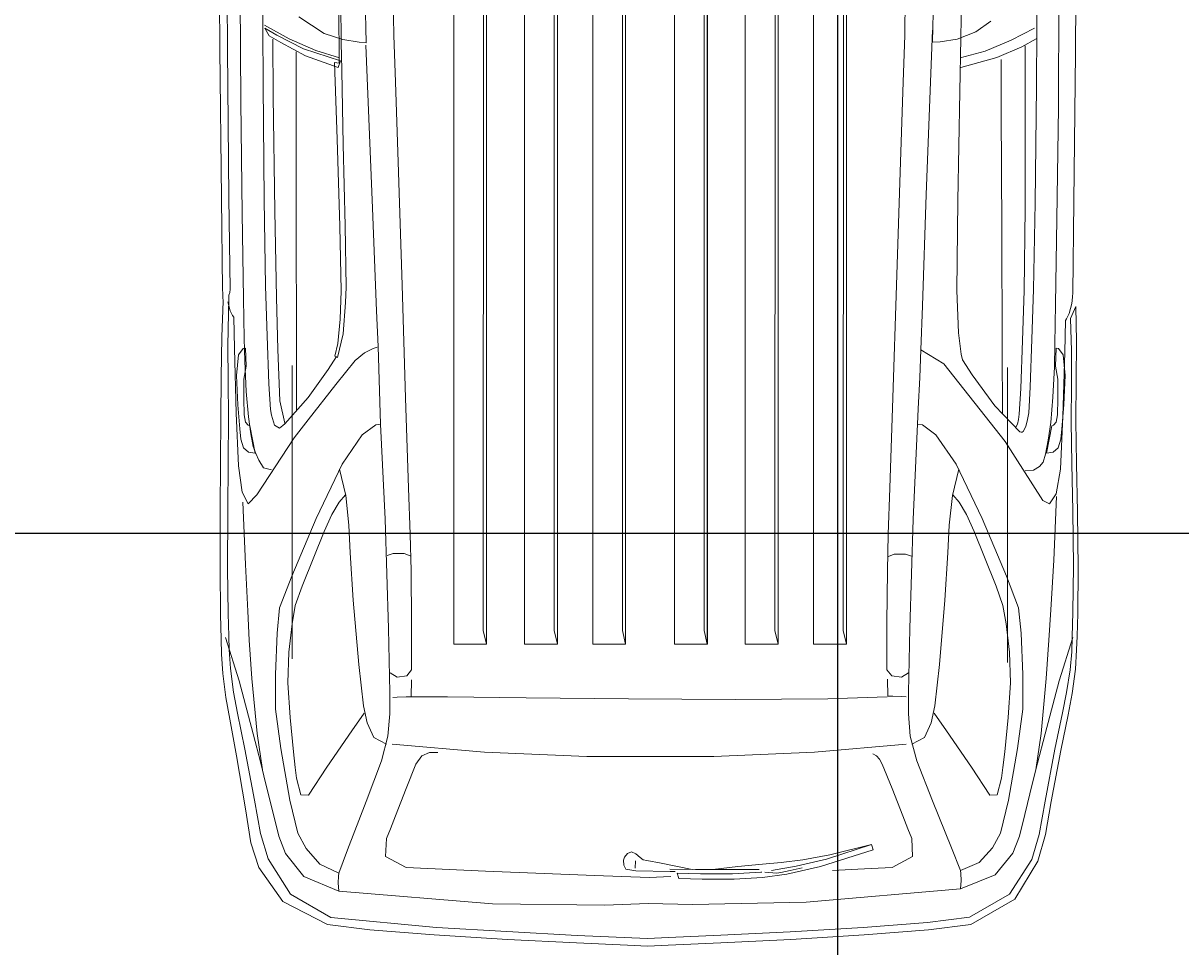
# Model space of a CAD drawing. Units: inches. Extents: x 37 to 706, y -568 to 110.
# Tile 11 of 24: x 444 to 494, y -468 to -428. Entities that reach past the tile are written whole.
import ezdxf

# ---------------------------------------------------------------- set-up
doc = ezdxf.new("R2010")
doc.units = ezdxf.units.IN
doc.header["$MEASUREMENT"] = 0
doc.layers.add('A-ANNO-DIMS', color=2, linetype='Continuous', lineweight=18)
doc.layers.add('A-SITE-VEHI', color=8, linetype='Continuous', lineweight=13)
doc.styles.get("Standard").update_dxf_attribs({"font": 'arial.ttf'})
doc.dimstyles.get("Standard").update_dxf_attribs({"dimtxt": 0.18, "dimasz": 0.18, "dimexe": 0.18, "dimexo": 0.0625, "dimgap": 0.09, "dimtad": 0, "dimtih": 1, "dimtoh": 1, "dimdec": 0, "dimzin": 0, "dimdsep": 46, "dimlunit": 3, "dimtxsty": 'Standard', "dimcen": 0.09, "dimadec": 0, "dimazin": 0, "dimtfac": 1, "dimtdec": 0, "dimtofl": 0, "dimtmove": 0, "dimatfit": 3, "dimfxl": 1, "dimtolj": 1, "dimtzin": 0, "dimarcsym": 0})

# ---------------------------------------------------------------- blocks, each defined once
blk = doc.blocks.new('CAR-SEDAN-PLAN')
for p, q in [((13.604, 13.133), (13.604, 50.661)), ((14.891, 13.73), (14.905, 50.543)), ((15.034, 50.661), (15.034, 13.133)), ((15.035, 50.661), (15.035, 13.133)), ((16.686, 13.133), (16.686, 50.661)), ((17.973, 13.73), (17.987, 50.543)), ((18.115, 50.661), (18.115, 13.133)), ((18.117, 50.661), (18.117, 13.133)), ((19.657, 13.133), (19.657, 50.661)), ((20.944, 13.73), (20.958, 50.543)), ((21.087, 50.661), (21.087, 13.133)), ((21.088, 50.661), (21.088, 13.133)), ((23.212, 13.133), (23.212, 50.661)), ((24.499, 13.73), (24.513, 50.543)), ((24.642, 50.661), (24.642, 13.133)), ((24.643, 50.661), (24.643, 13.133)), ((26.294, 13.133), (26.294, 50.661)), ((27.581, 13.73), (27.595, 50.543)), ((27.723, 50.661), (27.723, 13.133)), ((27.725, 50.661), (27.725, 13.133)), ((29.265, 13.133), (29.265, 50.661)), ((30.553, 13.73), (30.567, 50.543)), ((30.696, 50.661), (30.696, 13.133)), ((9.713, 43.414), (9.796, 39.289)), ((5.287, 43.269), (5.301, 39.967)), ((34.542, 43.262), (34.438, 39.318)), ((35.714, 43.262), (35.681, 39.496)), ((38.971, 43.074), (38.982, 39.925)), ((3.432, 39.004), (3.403, 42.392)), ((3.734, 42.392), (3.762, 39.007)), ((4.314, 41.922), (4.342, 36.731)), ((40.658, 38.847), (40.687, 42.232)), ((10.998, 39.61), (10.962, 41.449)), ((33.232, 39.61), (33.258, 41.449)), ((39.946, 41.674), (39.918, 36.482)), ((8.623, 38.413), (8.61, 40.812)), ((8.689, 40.947), (8.707, 39.376)), ((7.97, 39.706), (6.86, 40.42)), ((5.301, 39.967), (5.315, 37.467)), ((5.378, 40.068), (6.446, 39.47)), ((5.576, 39.596), (5.383, 39.926)), ((5.383, 39.926), (5.907, 39.624)), ((34.436, 39.852), (34.17, 32.694)), ((36.321, 39.78), (36.975, 40.234)), ((38.884, 39.936), (37.863, 39.414)), ((38.982, 39.925), (38.961, 37.396)), ((6.083, 39.306), (5.576, 39.596)), ((5.727, 39.459), (5.754, 36.963)), ((5.907, 39.624), (7.068, 39.031)), ((7.162, 38.735), (6.083, 39.306)), ((6.446, 39.47), (7.6, 38.961)), ((8.786, 39.439), (7.97, 39.706)), ((8.707, 39.376), (8.71, 39.215)), ((9.493, 39.318), (8.786, 39.439)), ((9.796, 39.289), (9.493, 39.318)), ((11.071, 37.604), (10.998, 39.61)), ((33.159, 37.604), (33.232, 39.61)), ((34.438, 39.318), (34.768, 39.333)), ((34.768, 39.333), (35.515, 39.45)), ((35.515, 39.45), (36.321, 39.78)), ((35.681, 39.496), (35.635, 37.18)), ((37.863, 39.414), (36.73, 38.932)), ((38.331, 39.125), (38.947, 39.462)), ((3.493, 32.542), (3.432, 39.004)), ((3.762, 39.007), (3.823, 32.551)), ((6.745, 38.908), (6.755, 31.469)), ((7.068, 39.031), (8.678, 38.516)), ((7.6, 38.961), (8.63, 38.647)), ((8.71, 39.215), (8.718, 38.766)), ((9.785, 39.195), (10.065, 32.102)), ((36.73, 38.932), (35.646, 38.643)), ((37.235, 38.651), (38.331, 39.125)), ((38.468, 39.17), (38.473, 36.823)), ((40.598, 32.392), (40.658, 38.847)), ((8.583, 38.221), (7.162, 38.735)), ((8.528, 35.109), (8.424, 38.44)), ((8.424, 38.44), (8.623, 38.413)), ((8.678, 38.516), (8.583, 38.221)), ((8.718, 38.766), (8.731, 38.071)), ((35.681, 38.217), (37.235, 38.651)), ((37.423, 38.564), (37.433, 36.292)), ((8.731, 38.071), (8.801, 34.877)), ((5.315, 37.467), (5.354, 32.465)), ((11.199, 33.662), (11.071, 37.604)), ((33.03, 33.662), (33.159, 37.604)), ((38.961, 37.396), (38.908, 32.341)), ((5.754, 36.963), (5.818, 31.97)), ((35.635, 37.18), (35.548, 32.425)), ((38.473, 36.823), (38.469, 32.105)), ((4.342, 36.731), (4.403, 31.875)), ((37.433, 36.292), (37.457, 31.221)), ((39.918, 36.482), (39.857, 31.627)), ((8.645, 31.317), (8.528, 35.109)), ((8.801, 34.877), (8.881, 31.335)), ((11.355, 28.753), (11.199, 33.662)), ((32.874, 28.753), (33.03, 33.662)), ((3.546, 28.561), (3.493, 32.542)), ((3.823, 32.551), (3.876, 28.574)), ((5.354, 32.465), (5.415, 28.71)), ((34.17, 32.694), (34.002, 27.855)), ((35.548, 32.425), (35.501, 28.522)), ((38.908, 32.341), (38.84, 28.558)), ((40.545, 28.416), (40.598, 32.392)), ((4.403, 31.875), (4.464, 28.172)), ((5.818, 31.97), (5.892, 28.219)), ((10.065, 32.102), (10.25, 27.635)), ((38.469, 32.105), (38.427, 28.503)), ((6.755, 31.469), (6.762, 26.153)), ((8.713, 28.508), (8.645, 31.317)), ((8.881, 31.335), (8.919, 28.667)), ((39.857, 31.627), (39.796, 27.924)), ((37.457, 31.221), (37.48, 25.971)), ((11.511, 23.847), (11.355, 28.753)), ((32.718, 23.847), (32.874, 28.753)), ((3.551, 28.393), (3.546, 28.561)), ((3.558, 28.225), (3.551, 28.393)), ((3.579, 28.059), (3.558, 28.225)), ((3.819, 28.315), (3.815, 28.178)), ((3.856, 28.436), (3.819, 28.315)), ((3.876, 28.574), (3.856, 28.436)), ((5.415, 28.71), (5.486, 26.554)), ((5.892, 28.219), (5.946, 25.954)), ((8.671, 27.267), (8.713, 28.508)), ((8.919, 28.667), (8.894, 27.992)), ((35.501, 28.522), (35.566, 26.682)), ((38.427, 28.503), (38.356, 26.347)), ((38.84, 28.558), (38.769, 26.402)), ((40.519, 28.091), (40.535, 28.246)), ((40.535, 28.246), (40.545, 28.416)), ((3.52, 26.505), (3.579, 28.059)), ((3.88, 27.64), (3.771, 28.026)), ((3.815, 28.178), (3.801, 27.531)), ((4.464, 28.172), (4.492, 26.437)), ((8.894, 27.992), (8.788, 26.636)), ((34.002, 27.855), (33.939, 25.939)), ((39.796, 27.924), (39.768, 26.188)), ((40.387, 27.519), (40.498, 27.951)), ((40.449, 27.298), (40.675, 27.828)), ((40.498, 27.951), (40.519, 28.091)), ((40.675, 27.828), (40.709, 26.308)), ((3.801, 27.531), (3.77, 26.116)), ((3.984, 27.426), (3.88, 27.64)), ((4.03, 27.36), (3.984, 27.426)), ((4.062, 25.992), (4.03, 27.36)), ((8.558, 26.208), (8.671, 27.267)), ((10.25, 27.635), (10.317, 26.081)), ((40.194, 25.84), (40.225, 27.208)), ((40.225, 27.208), (40.276, 27.281)), ((40.276, 27.281), (40.387, 27.519)), ((40.488, 25.901), (40.449, 27.298)), ((3.484, 24.748), (3.52, 26.505)), ((4.492, 26.437), (4.514, 25.45)), ((5.486, 26.554), (5.557, 24.461)), ((8.437, 25.661), (8.558, 26.208)), ((8.788, 26.636), (8.548, 25.606)), ((35.566, 26.682), (35.686, 25.757)), ((38.356, 26.347), (38.285, 24.254)), ((38.769, 26.402), (38.698, 24.309)), ((40.709, 26.308), (40.697, 24.613)), ((3.77, 26.116), (3.787, 24.613)), ((4.141, 23.187), (4.062, 25.992)), ((4.24, 25.718), (4.151, 24.827)), ((4.44, 26.001), (4.24, 25.718)), ((4.551, 26.018), (4.44, 26.001)), ((4.571, 25.221), (4.551, 26.018)), ((5.946, 25.954), (6.033, 23.727)), ((6.762, 26.153), (6.765, 23.311)), ((9.729, 25.804), (9.322, 25.478)), ((10.107, 25.994), (9.729, 25.804)), ((10.273, 26.055), (10.107, 25.994)), ((10.317, 26.081), (10.426, 22.71)), ((33.939, 25.939), (33.885, 24.736)), ((33.939, 25.939), (34.933, 25.326)), ((35.686, 25.757), (35.75, 25.503)), ((37.48, 25.971), (37.49, 23.159)), ((39.768, 26.188), (39.746, 25.202)), ((39.796, 25.221), (39.816, 26.018)), ((39.816, 26.018), (39.928, 26.001)), ((39.928, 26.001), (40.128, 25.718)), ((40.115, 23.036), (40.194, 25.84)), ((40.128, 25.718), (40.217, 24.827)), ((40.485, 24.433), (40.488, 25.901)), ((4.47, 24.664), (4.571, 25.221)), ((4.514, 25.45), (4.576, 24.132)), ((6.579, 25.262), (6.579, 12.495)), ((8.505, 25.655), (8.139, 25.088)), ((8.548, 25.606), (8.437, 25.661)), ((9.322, 25.478), (8.474, 24.429)), ((34.933, 25.326), (37.597, 21.952)), ((35.75, 25.503), (36.174, 24.851)), ((39.746, 25.202), (39.684, 23.884)), ((39.897, 24.664), (39.796, 25.221)), ((3.472, 22.96), (3.484, 24.748)), ((4.151, 24.827), (4.216, 23.545)), ((8.139, 25.088), (7.271, 23.868)), ((33.885, 24.736), (33.823, 23.365)), ((36.174, 24.851), (37.15, 23.504)), ((37.699, 25.17), (37.699, 12.334)), ((40.217, 24.827), (40.151, 23.545)), ((3.787, 24.613), (3.803, 22.96)), ((4.466, 23.8), (4.47, 24.664)), ((5.557, 24.461), (5.628, 23.347)), ((8.474, 24.429), (7.27, 22.892)), ((38.285, 24.254), (38.214, 23.14)), ((38.698, 24.309), (38.627, 23.195)), ((39.901, 23.8), (39.897, 24.664)), ((40.477, 22.799), (40.485, 24.433)), ((40.697, 24.613), (40.683, 22.854)), ((4.482, 23.116), (4.466, 23.8)), ((4.576, 24.132), (4.669, 23.027)), ((6.033, 23.727), (6.25, 22.744)), ((7.271, 23.868), (6.252, 22.718)), ((11.64, 19.914), (11.511, 23.847)), ((32.59, 19.914), (32.718, 23.847)), ((39.684, 23.884), (39.591, 22.779)), ((39.885, 23.116), (39.901, 23.8)), ((4.243, 20.896), (4.141, 23.187)), ((4.216, 23.545), (4.303, 22.495)), ((5.628, 23.347), (5.675, 23.096)), ((33.823, 23.365), (33.793, 22.71)), ((37.15, 23.504), (38.236, 22.378)), ((38.627, 23.195), (38.57, 22.906)), ((40.151, 23.545), (40.064, 22.495)), ((3.463, 21.075), (3.472, 22.96)), ((3.803, 22.96), (3.793, 21.075)), ((4.546, 22.789), (4.482, 23.116)), ((4.666, 22.658), (4.546, 22.789)), ((4.669, 23.027), (4.776, 22.289)), ((5.675, 23.096), (5.809, 22.664)), ((6.173, 22.65), (6.252, 22.718)), ((7.27, 22.892), (6.658, 22.104)), ((10.426, 22.71), (10.213, 22.669)), ((10.426, 22.71), (10.623, 18.569)), ((33.793, 22.71), (33.596, 18.569)), ((33.793, 22.71), (34.007, 22.669)), ((38.142, 22.707), (38.056, 22.552)), ((38.178, 22.908), (38.142, 22.707)), ((38.214, 23.14), (38.178, 22.908)), ((38.57, 22.906), (38.496, 22.598)), ((39.591, 22.779), (39.479, 22.007)), ((39.702, 22.658), (39.821, 22.789)), ((39.821, 22.789), (39.885, 23.116)), ((40.012, 20.744), (40.115, 23.036)), ((40.502, 20.982), (40.477, 22.799)), ((40.683, 22.854), (40.709, 20.996)), ((4.303, 22.495), (4.347, 22.059)), ((4.73, 22.634), (4.666, 22.658)), ((4.964, 21.437), (4.73, 22.634)), ((4.776, 22.289), (4.883, 21.74)), ((5.809, 22.664), (6.019, 22.53)), ((6.019, 22.53), (6.095, 22.587)), ((6.095, 22.587), (6.173, 22.65)), ((9.627, 22.239), (8.747, 20.959)), ((10.213, 22.669), (9.627, 22.239)), ((34.007, 22.669), (34.593, 22.239)), ((34.593, 22.239), (35.473, 20.959)), ((38.236, 22.378), (38.293, 22.351)), ((38.293, 22.351), (38.344, 22.355)), ((38.344, 22.355), (38.389, 22.385)), ((38.496, 22.598), (38.389, 22.385)), ((39.404, 21.437), (39.637, 22.634)), ((39.637, 22.634), (39.702, 22.658)), ((40.064, 22.495), (40.02, 22.059)), ((4.347, 22.059), (4.458, 21.676)), ((4.458, 21.676), (4.673, 21.491)), ((4.883, 21.74), (4.989, 21.429)), ((6.658, 22.104), (5.04, 19.635)), ((37.597, 21.952), (39.239, 19.387)), ((39.479, 22.007), (39.364, 21.397)), ((39.909, 21.676), (39.695, 21.491)), ((40.02, 22.059), (39.909, 21.676)), ((4.673, 21.491), (4.964, 21.437)), ((4.989, 21.429), (5.122, 21.136)), ((39.364, 21.397), (39.252, 21.052)), ((39.695, 21.491), (39.404, 21.437)), ((3.446, 18.903), (3.463, 21.075)), ((3.793, 21.075), (3.776, 18.903)), ((4.396, 19.749), (4.243, 20.896)), ((5.122, 21.136), (5.335, 20.805)), ((5.335, 20.805), (5.672, 20.722)), ((8.747, 20.959), (7.622, 18.6)), ((8.64, 20.745), (8.911, 19.602)), ((35.58, 20.745), (35.309, 19.602)), ((35.473, 20.959), (36.598, 18.6)), ((38.843, 20.707), (38.468, 20.681)), ((39.099, 20.862), (38.843, 20.707)), ((39.252, 21.052), (39.099, 20.862)), ((39.822, 19.677), (40.012, 20.744)), ((40.548, 18.939), (40.502, 20.982)), ((40.709, 20.996), (40.757, 18.876)), ((4.655, 19.245), (4.396, 19.749)), ((11.712, 17.922), (11.64, 19.914)), ((32.517, 17.922), (32.59, 19.914)), ((39.532, 19.233), (39.822, 19.677)), ((4.434, 19.305), (4.545, 16.6)), ((5.04, 19.635), (4.655, 19.245)), ((8.625, 19.316), (8.297, 18.78)), ((8.89, 19.637), (8.625, 19.316)), ((8.911, 19.602), (9.047, 18.315)), ((35.309, 19.602), (35.172, 18.315)), ((35.33, 19.637), (35.595, 19.316)), ((35.595, 19.316), (35.923, 18.78)), ((39.239, 19.387), (39.532, 19.233)), ((39.844, 19.553), (39.718, 16.784)), ((3.437, 16.422), (3.446, 18.903)), ((3.776, 18.903), (3.767, 16.422)), ((8.297, 18.78), (7.961, 18.03)), ((35.923, 18.78), (36.259, 18.03)), ((40.573, 16.526), (40.548, 18.939)), ((40.757, 18.876), (40.783, 16.422)), ((7.622, 18.6), (6.561, 16.09)), ((9.047, 18.315), (9.104, 17.101)), ((10.623, 18.569), (10.765, 13.809)), ((33.596, 18.569), (33.455, 13.809)), ((35.172, 18.315), (35.115, 17.101)), ((36.598, 18.6), (37.659, 16.09)), ((7.961, 18.03), (7.517, 16.918)), ((11.752, 16.319), (11.712, 17.922)), ((32.477, 16.319), (32.517, 17.922)), ((36.259, 18.03), (36.702, 16.918)), ((7.517, 16.918), (7.011, 15.663)), ((9.104, 17.101), (9.236, 15.044)), ((10.707, 16.994), (10.967, 17.077)), ((10.967, 17.077), (11.449, 17.073)), ((11.449, 17.073), (11.705, 16.973)), ((32.78, 17.046), (32.525, 16.946)), ((33.262, 17.05), (32.78, 17.046)), ((33.522, 16.966), (33.262, 17.05)), ((35.115, 17.101), (34.983, 15.044)), ((36.702, 16.918), (37.209, 15.663)), ((39.718, 16.784), (39.589, 14.629)), ((3.453, 14.417), (3.437, 16.422)), ((3.767, 16.422), (3.785, 14.465)), ((4.545, 16.6), (4.646, 14.565)), ((11.771, 14.081), (11.752, 16.319)), ((32.458, 14.081), (32.477, 16.319)), ((40.555, 14.519), (40.573, 16.526)), ((40.783, 16.422), (40.764, 14.465)), ((6.561, 16.09), (6.031, 14.707)), ((7.011, 15.663), (6.71, 14.814)), ((37.209, 15.663), (37.509, 14.814)), ((37.659, 16.09), (38.188, 14.707)), ((6.031, 14.707), (5.922, 13.615)), ((6.71, 14.814), (6.571, 14.015)), ((9.236, 15.044), (9.472, 12.249)), ((34.983, 15.044), (34.748, 12.249)), ((37.509, 14.814), (37.648, 14.015)), ((38.188, 14.707), (38.298, 13.615)), ((39.589, 14.629), (39.51, 13.313)), ((3.483, 13.349), (3.453, 14.417)), ((3.785, 14.465), (3.82, 13.484)), ((4.646, 14.565), (4.709, 13.313)), ((40.522, 13.447), (40.555, 14.519)), ((40.764, 14.465), (40.73, 13.484)), ((5.922, 13.615), (5.844, 11.809)), ((6.571, 14.015), (6.432, 12.779)), ((10.765, 13.809), (10.819, 11.026)), ((11.772, 12.018), (11.771, 14.081)), ((15.034, 13.133), (14.891, 13.73)), ((18.115, 13.133), (17.973, 13.73)), ((21.087, 13.133), (20.944, 13.73)), ((24.642, 13.133), (24.499, 13.73)), ((27.723, 13.133), (27.581, 13.73)), ((30.696, 13.133), (30.553, 13.73)), ((32.458, 12.018), (32.458, 14.081)), ((33.455, 13.809), (33.4, 11.026)), ((37.648, 14.015), (37.787, 12.779)), ((38.298, 13.615), (38.376, 11.809)), ((3.499, 12.702), (3.483, 13.349)), ((3.673, 13.421), (4.262, 11.543)), ((3.82, 13.484), (3.838, 12.885)), ((4.709, 13.313), (4.826, 11.635)), ((15.035, 13.133), (13.604, 13.133)), ((18.117, 13.133), (16.686, 13.133)), ((21.088, 13.133), (19.657, 13.133)), ((24.643, 13.133), (23.212, 13.133)), ((27.725, 13.133), (26.294, 13.133)), ((30.696, 13.133), (29.265, 13.133)), ((39.51, 13.313), (39.394, 11.635)), ((40.546, 13.421), (39.958, 11.543)), ((40.504, 12.798), (40.522, 13.447)), ((40.73, 13.484), (40.711, 12.885)), ((3.552, 11.862), (3.499, 12.702)), ((3.838, 12.885), (3.891, 12.073)), ((6.432, 12.779), (6.389, 11.455)), ((37.787, 12.779), (37.831, 11.455)), ((40.436, 12.011), (40.504, 12.798)), ((40.711, 12.885), (40.658, 12.044)), ((9.472, 12.249), (9.676, 10.455)), ((34.748, 12.249), (34.544, 10.455)), ((3.686, 10.809), (3.552, 11.862)), ((3.891, 12.073), (4.021, 11.046)), ((4.826, 11.635), (5.045, 9.251)), ((5.844, 11.809), (5.853, 10.312)), ((10.833, 11.88), (11.14, 11.695)), ((11.14, 11.695), (11.56, 11.754)), ((11.56, 11.754), (11.772, 12.018)), ((32.669, 11.754), (32.458, 12.018)), ((32.479, 11.611), (32.503, 10.878)), ((33.089, 11.695), (32.669, 11.754)), ((33.396, 11.88), (33.089, 11.695)), ((38.376, 11.809), (38.367, 10.312)), ((39.394, 11.635), (39.174, 9.251)), ((40.277, 11.029), (40.436, 12.011)), ((40.658, 12.044), (40.524, 10.992)), ((4.262, 11.543), (4.883, 9.236)), ((6.389, 11.455), (6.488, 9.945)), ((11.772, 11.581), (11.748, 10.848)), ((37.831, 11.455), (37.732, 9.945)), ((39.958, 11.543), (39.337, 9.236)), ((3.861, 9.877), (3.686, 10.809)), ((4.021, 11.046), (4.191, 10.136)), ((10.819, 11.026), (10.822, 10.099)), ((11.15, 10.821), (10.962, 10.812)), ((11.536, 10.839), (11.15, 10.821)), ((11.748, 10.848), (11.536, 10.839)), ((13.334, 10.84), (11.748, 10.848)), ((16.76, 10.8), (13.334, 10.84)), ((21.205, 10.754), (16.76, 10.8)), ((25.852, 10.729), (21.205, 10.754)), ((29.881, 10.751), (25.852, 10.729)), ((32.471, 10.848), (29.881, 10.751)), ((32.503, 10.878), (32.714, 10.869)), ((32.714, 10.869), (33.101, 10.852)), ((33.101, 10.852), (33.289, 10.843)), ((33.4, 11.026), (33.398, 10.099)), ((40.092, 10.143), (40.277, 11.029)), ((40.524, 10.992), (40.35, 10.059)), ((4.191, 10.136), (4.515, 8.572)), ((5.853, 10.312), (6.079, 8.596)), ((9.169, 9.358), (9.711, 10.133)), ((9.676, 10.455), (9.84, 9.71)), ((10.822, 10.099), (10.745, 9.132)), ((33.398, 10.099), (33.475, 9.132)), ((34.544, 10.455), (34.38, 9.71)), ((35.051, 9.358), (34.508, 10.133)), ((38.367, 10.312), (38.141, 8.596)), ((39.767, 8.563), (40.092, 10.143)), ((4.16, 8.275), (3.861, 9.877)), ((6.488, 9.945), (6.635, 8.451)), ((9.84, 9.71), (10.131, 9.068)), ((34.38, 9.71), (34.089, 9.068)), ((37.732, 9.945), (37.585, 8.451)), ((40.35, 10.059), (40.028, 8.506)), ((4.883, 9.236), (5.21, 7.954)), ((5.045, 9.251), (5.281, 7.668)), ((8.087, 7.788), (9.169, 9.358)), ((10.745, 9.132), (10.462, 8.061)), ((33.475, 9.132), (33.758, 8.061)), ((36.133, 7.788), (35.051, 9.358)), ((39.174, 9.251), (38.939, 7.668)), ((39.337, 9.236), (39.01, 7.954)), ((4.515, 8.572), (4.943, 6.346)), ((6.079, 8.596), (6.472, 6.347)), ((10.131, 9.068), (10.676, 8.776)), ((14.948, 8.438), (10.926, 8.776)), ((33.293, 8.776), (29.309, 8.438)), ((34.089, 9.068), (33.543, 8.776)), ((38.141, 8.596), (37.748, 6.347)), ((4.542, 5.974), (4.16, 8.275)), ((6.635, 8.451), (6.71, 7.775)), ((10.462, 8.061), (9.79, 6.285)), ((11.963, 7.918), (12.22, 8.276)), ((12.22, 8.276), (12.546, 8.416)), ((12.546, 8.416), (12.908, 8.42)), ((19.398, 8.244), (14.948, 8.438)), ((22.181, 8.24), (19.398, 8.244)), ((24.927, 8.244), (22.181, 8.24)), ((29.309, 8.438), (24.927, 8.244)), ((31.842, 8.368), (31.999, 8.276)), ((31.999, 8.276), (32.139, 8.129)), ((32.139, 8.129), (32.257, 7.918)), ((33.758, 8.061), (34.442, 6.313)), ((37.585, 8.451), (37.509, 7.775)), ((39.34, 6.307), (39.767, 8.563)), ((40.028, 8.506), (39.603, 6.295)), ((5.21, 7.954), (5.421, 7.098)), ((6.71, 7.775), (6.771, 7.309)), ((7.282, 6.56), (8.087, 7.788)), ((11.533, 6.853), (11.963, 7.918)), ((32.257, 7.918), (32.687, 6.853)), ((36.938, 6.56), (36.133, 7.788)), ((37.509, 7.775), (37.448, 7.309)), ((39.01, 7.954), (38.798, 7.098)), ((5.421, 7.098), (5.76, 5.725)), ((6.771, 7.309), (6.959, 6.574)), ((37.448, 7.309), (37.261, 6.574)), ((38.798, 7.098), (38.459, 5.725)), ((6.959, 6.574), (7.282, 6.56)), ((11.071, 5.66), (11.533, 6.853)), ((32.687, 6.853), (33.149, 5.66)), ((37.261, 6.574), (36.938, 6.56)), ((4.943, 6.346), (5.195, 4.901)), ((6.472, 6.347), (6.817, 4.917)), ((9.79, 6.285), (8.99, 4.184)), ((34.442, 6.313), (35.263, 4.266)), ((37.748, 6.347), (37.402, 4.917)), ((39.087, 4.847), (39.34, 6.307)), ((39.603, 6.295), (39.352, 4.86)), ((4.77, 4.491), (4.542, 5.974)), ((5.76, 5.725), (5.996, 4.774)), ((10.855, 5.095), (11.071, 5.66)), ((33.149, 5.66), (33.365, 5.095)), ((38.459, 5.725), (38.224, 4.774)), ((10.674, 4.684), (10.855, 5.095)), ((33.365, 5.095), (33.546, 4.684)), ((5.195, 4.901), (5.531, 3.798)), ((5.996, 4.774), (6.288, 4.02)), ((6.817, 4.917), (7.185, 4.242)), ((10.643, 3.899), (10.674, 4.684)), ((33.546, 4.684), (33.576, 3.899)), ((37.402, 4.917), (37.046, 4.27)), ((38.224, 4.774), (37.943, 4.048)), ((38.757, 3.761), (39.087, 4.847)), ((39.352, 4.86), (39.023, 3.695)), ((5.125, 3.422), (4.77, 4.491)), ((7.185, 4.242), (7.784, 3.56)), ((8.99, 4.184), (8.604, 3.17)), ((21.034, 3.871), (21.162, 4.032)), ((21.162, 4.032), (21.341, 4.104)), ((21.341, 4.104), (21.538, 4.014)), ((29.573, 3.454), (31.866, 4.183)), ((31.793, 4.421), (29.822, 3.785)), ((31.793, 4.421), (29.98, 3.966)), ((31.866, 4.183), (31.793, 4.421)), ((35.263, 4.266), (35.662, 3.281)), ((37.046, 4.27), (36.47, 3.641)), ((37.943, 4.048), (37.164, 3.102)), ((5.531, 3.798), (6.501, 2.261)), ((6.288, 4.02), (7.089, 3.02)), ((7.784, 3.56), (8.604, 3.17)), ((11.534, 3.416), (10.643, 3.899)), ((20.997, 3.733), (21.034, 3.871)), ((21.004, 3.524), (20.997, 3.733)), ((21.499, 3.391), (21.521, 3.714)), ((21.538, 4.014), (21.716, 3.853)), ((21.716, 3.853), (21.845, 3.754)), ((22.004, 3.727), (21.845, 3.754)), ((22.637, 3.606), (22.004, 3.727)), ((23.982, 3.332), (22.637, 3.606)), ((27.049, 3.559), (25.968, 3.461)), ((27.853, 3.637), (27.049, 3.559)), ((28.803, 3.753), (27.853, 3.637)), ((29.822, 3.785), (28.511, 3.471)), ((29.98, 3.966), (28.803, 3.753)), ((33.576, 3.899), (32.686, 3.416)), ((36.47, 3.641), (35.662, 3.281)), ((37.799, 2.256), (38.757, 3.761)), ((39.023, 3.695), (38.022, 2.04)), ((6.173, 1.944), (5.125, 3.422)), ((8.588, 3.046), (8.572, 2.747)), ((8.604, 3.17), (8.588, 3.046)), ((14.99, 3.257), (11.534, 3.416)), ((19.725, 3.075), (14.99, 3.257)), ((22.11, 2.987), (19.725, 3.075)), ((21.096, 3.341), (21.004, 3.524)), ((21.524, 3.276), (21.096, 3.341)), ((23.024, 3.239), (21.524, 3.276)), ((24.129, 3.334), (23.01, 3.34)), ((23.236, 3.237), (23.024, 3.239)), ((24.339, 3.147), (23.324, 3.177)), ((23.324, 3.177), (23.396, 2.94)), ((25.943, 3.33), (24.129, 3.334)), ((25.734, 3.146), (24.339, 3.147)), ((25.968, 3.461), (24.882, 3.334)), ((26.968, 3.215), (25.734, 3.146)), ((26.893, 3.328), (25.943, 3.33)), ((26.981, 3.216), (26.968, 3.215)), ((26.995, 3.218), (26.981, 3.216)), ((27.01, 3.22), (26.995, 3.218)), ((27.04, 2.977), (28.095, 3.12)), ((27.673, 3.169), (27.15, 3.209)), ((28.511, 3.471), (27.428, 3.283)), ((27.835, 3.2), (27.673, 3.169)), ((28.24, 3.283), (27.835, 3.2)), ((28.095, 3.12), (29.573, 3.454)), ((28.765, 3.406), (28.24, 3.283)), ((31.193, 3.34), (30.088, 3.293)), ((32.083, 3.382), (31.193, 3.34)), ((32.686, 3.416), (32.083, 3.382)), ((35.662, 3.281), (35.678, 3.156)), ((37.164, 3.102), (35.662, 2.494)), ((35.678, 3.156), (35.694, 2.857)), ((7.089, 3.02), (8.604, 2.384)), ((8.572, 2.747), (8.604, 2.384)), ((23.061, 3.022), (22.11, 2.987)), ((23.396, 2.94), (24.411, 2.909)), ((24.411, 2.909), (25.806, 2.909)), ((25.806, 2.909), (27.04, 2.977)), ((35.694, 2.857), (35.662, 2.494)), ((6.501, 2.261), (8.259, 1.242)), ((15.288, 1.831), (8.604, 2.384)), ((35.662, 2.494), (28.947, 1.913)), ((36.048, 1.256), (37.799, 2.256)), ((38.022, 2.04), (36.112, 0.932)), ((8.107, 0.932), (6.173, 1.944)), ((20.178, 1.778), (15.288, 1.831)), ((22.074, 1.844), (20.178, 1.778)), ((24.001, 1.806), (22.074, 1.844)), ((28.947, 1.913), (24.001, 1.806)), ((8.259, 1.242), (12.855, 0.801)), ((31.426, 0.81), (34.217, 1.026)), ((34.217, 1.026), (36.048, 1.256)), ((9.948, 0.701), (8.107, 0.932)), ((12.757, 0.482), (9.948, 0.701)), ((12.855, 0.801), (18.978, 0.464)), ((25.227, 0.467), (28.251, 0.62)), ((28.251, 0.62), (31.426, 0.81)), ((34.271, 0.701), (31.463, 0.482)), ((36.112, 0.932), (34.271, 0.701)), ((15.951, 0.29), (12.757, 0.482)), ((18.943, 0.137), (15.951, 0.29)), ((21.163, 0.036), (18.943, 0.137)), ((18.978, 0.464), (22.045, 0.33)), ((22.032, 0), (21.163, 0.036)), ((22.941, 0.036), (22.032, 0)), ((22.045, 0.33), (22.946, 0.366)), ((25.236, 0.137), (22.941, 0.036)), ((22.946, 0.366), (25.227, 0.467)), ((28.269, 0.29), (25.236, 0.137)), ((31.463, 0.482), (28.269, 0.29))]:
    blk.add_line(p, q)
blk = doc.blocks.new('*D45')
at = {"layer": 'A-ANNO-DIMS', "color": 0, "lineweight": -2, "transparency": 16777216}
for p, q in [((88.021, -449.708), (705.888, -449.708)), ((705.708, -449.888), (705.708, -481.527)), ((705.708, -513.528), (705.708, -481.89)), ((79.021, -513.708), (705.888, -513.708))]:
    blk.add_line(p, q, dxfattribs=at)
at = {"layer": 'A-ANNO-DIMS', "color": 0, "transparency": 16777216}
for points in [[(705.678, -449.888), (705.738, -449.888), (705.708, -449.708)], [(705.678, -513.528), (705.738, -513.528), (705.708, -513.708)]]:
    blk.add_solid(points, dxfattribs=at)
at = {"layer": 'Defpoints', "color": 0, "transparency": 16777216}
for p in [(87.958, -449.708), (705.708, -449.708), (78.958, -513.708)]:
    blk.add_point(p, dxfattribs=at)
at = {"layer": 'A-ANNO-DIMS', "color": 0, "transparency": 16777216, "insert": (705.708, -481.708), "char_height": 0.18, "attachment_point": 5}
blk.add_mtext('\\A1;5\'-4"', dxfattribs=at)
blk = doc.blocks.new('*D63')
at = {"layer": 'A-ANNO-DIMS', "color": 0, "lineweight": -2, "transparency": 16777216}
for p, q in [((478.958, -142.771), (478.958, -567.638)), ((502.958, -151.771), (502.958, -567.638)), ((479.138, -567.458), (490.628, -567.458)), ((502.778, -567.458), (491.289, -567.458))]:
    blk.add_line(p, q, dxfattribs=at)
at = {"layer": 'A-ANNO-DIMS', "color": 0, "transparency": 16777216}
for points in [[(479.138, -567.428), (479.138, -567.488), (478.958, -567.458)], [(502.778, -567.428), (502.778, -567.488), (502.958, -567.458)]]:
    blk.add_solid(points, dxfattribs=at)
at = {"layer": 'Defpoints', "color": 0, "transparency": 16777216}
for p in [(478.958, -142.708), (502.958, -151.708), (502.958, -567.458)]:
    blk.add_point(p, dxfattribs=at)
at = {"layer": 'A-ANNO-DIMS', "color": 0, "transparency": 16777216, "insert": (490.958, -567.458), "char_height": 0.18, "attachment_point": 5}
blk.add_mtext('\\A1;2\'-0"', dxfattribs=at)

msp = doc.modelspace()

# ---------------------------------------------------------------- block references
at = {"layer": 'A-SITE-VEHI'}
msp.add_blockref('CAR-SEDAN-PLAN', (448.648, -467.674), dxfattribs=at)

# ---------------------------------------------------------------- dimensions: what is measured, and where the dimension line sits
at = {"layer": 'A-ANNO-DIMS'}
dim = msp.add_linear_dim(base=(502.958, -567.458), p1=(478.958, -142.708), p2=(502.958, -151.708), dimstyle='Standard', override={"dimdec": 1, "dimlfac": 1, "dimrnd": 0, "dimzin": 1, "dimdsep": 46, "dimlunit": 4, "dimfrac": 2}, dxfattribs=at)
dim.commit()
dim.dimension.update_dxf_attribs({"geometry": '*D63', "text_midpoint": (490.958, -567.458)})
dim = msp.add_linear_dim(base=(705.708, -449.708), p1=(78.958, -513.708), p2=(87.958, -449.708), angle=90, dimstyle='Standard', override={"dimdec": 1, "dimlfac": 1, "dimrnd": 0, "dimzin": 1, "dimdsep": 46, "dimlunit": 4, "dimfrac": 2}, dxfattribs=at)
dim.commit()
dim.dimension.update_dxf_attribs({"geometry": '*D45', "text_midpoint": (705.708, -481.708)})

doc.saveas('drawing.dxf')
